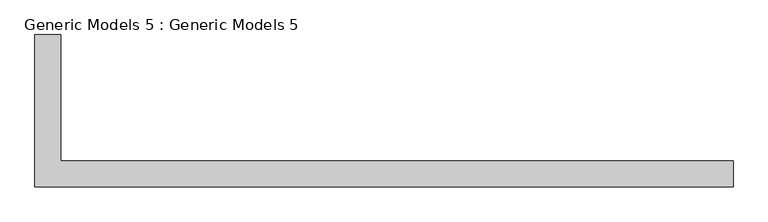
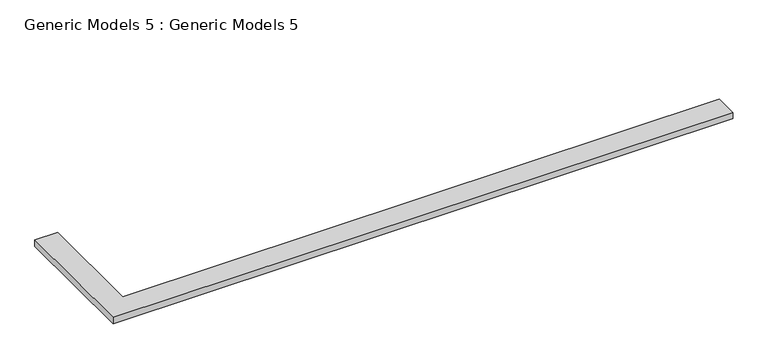
"""IFC4 building model written with IfcOpenShell, lengths in millimetres: proxy geometry, Generic Models 5 : Generic Models 5."""

from ifc_helpers import new_model, si_unit, frame, origin, place, context, project, spatial, polyline, outline, extrude, source, transform, mapped, element, save


def generic_models_5_generic_models_5_f772a959(model_context):
    return source(origin(), model_context, "Body", "SweptSolid", [
        extrude(outline(polyline([(3357.0521331, -11975.7643494), (3357.0521331, -12826.6643494), (7881.4271331, -12826.6643494), (7881.4271331, -13001.2893494), (3182.4271331, -13001.2893494), (3182.4271331, -11975.7643494), (3357.0521331, -11975.7643494)])), frame((0.0, 0.0, 4749.8), z_axis=(0.0, 0.0, 1.0), x_axis=(1.0, 0.0, 0.0)), (0.0, 0.0, 1.0), 50.8),
    ])


if __name__ == "__main__":
    model = new_model("IFC4")
    model_context = context("Model", 3, world=origin())
    ifc_project = project(units=[si_unit("LENGTHUNIT", "METRE", prefix="MILLI")], contexts=[model_context])
    site = spatial("IfcSite", under=ifc_project)
    building = spatial("IfcBuilding", under=site)
    placement = place(None, origin())
    generic_models_5_generic_models_5_shape = generic_models_5_generic_models_5_f772a959(model_context)
    element("IfcBuildingElementProxy", 1, Name="Generic Models 5 : Generic Models 5", ObjectType="Generic Models 5 : Generic Models 5", at=placement, inside=building, context=model_context, shape_type="MappedRepresentation", body=[
        mapped(generic_models_5_generic_models_5_shape, transform((0.0, 0.0, 0.0), x_axis=(1.0, 0.0, 0.0), y_axis=(0.0, 1.0, 0.0), z_axis=(0.0, 0.0, 1.0))),
    ])
    save(model, "model.ifc")
